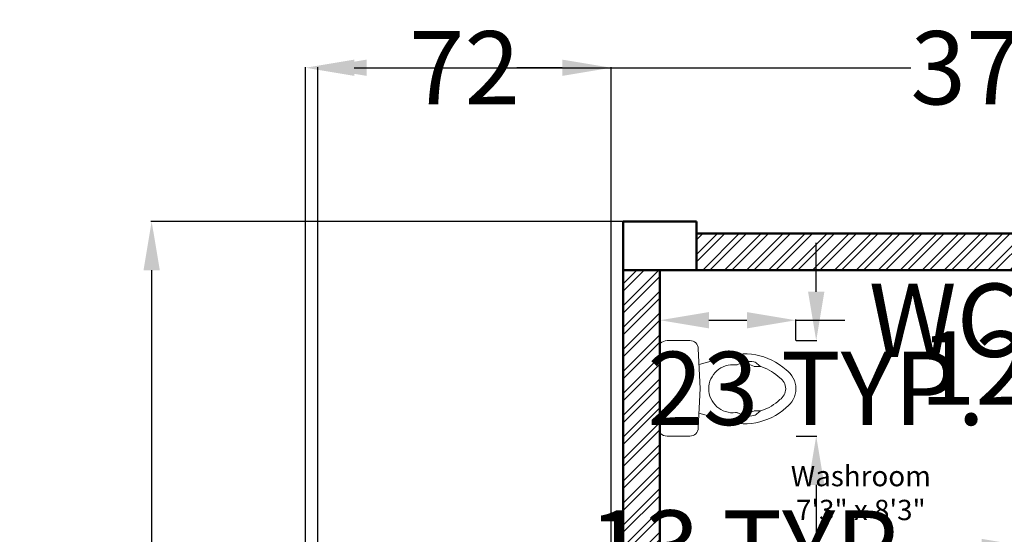
# Model space of a CAD drawing. Units: inches. Extents: x -90 to 536, y -553 to 299.
# Tile 21 of 27: x -35 to 207, y 173 to 299. Entities that reach past the tile are written whole.
import ezdxf

# ---------------------------------------------------------------- set-up
doc = ezdxf.new("R2010")
doc.units = ezdxf.units.IN
for name, color, linetype, lineweight in [('A-ANNO-DIMS', 2, 'Continuous', 18), ('A-AREA-IDEN', 7, 'Continuous', 18), ('A-COLS', 7, 'Continuous', 50), ('A-FLOR-FIXT', 8, 'Continuous', 18), ('A-WALL-PATT', 252, 'Continuous', 13), ('Outer Wall', 1, 'Continuous', 50)]:
    doc.layers.add(name, color=color, linetype=linetype, lineweight=lineweight)
doc.styles.get("Standard").update_dxf_attribs({"font": 'arial.ttf'})
doc.dimstyles.get("Standard").update_dxf_attribs({"dimtxt": 18, "dimasz": 12, "dimexe": 0.18, "dimexo": 0.0625, "dimgap": 0.09, "dimtad": 0, "dimtih": 1, "dimtoh": 1, "dimdec": 0, "dimzin": 0, "dimdsep": 46, "dimlunit": 3, "dimtxsty": 'Standard', "dimcen": 0.09, "dimadec": 0, "dimazin": 0, "dimtfac": 1, "dimtdec": 0, "dimtofl": 0, "dimtmove": 0, "dimatfit": 3, "dimfxl": 1, "dimtolj": 1, "dimtzin": 0, "dimarcsym": 0})

# ---------------------------------------------------------------- blocks, each defined once
blk = doc.blocks.new('A$C1308471B')
at = {"ltscale": 20}
for p, q in [((0, 0.4607), (0, 0.0186)), ((0.0354, 0.4793), (0.1495, 0.4793)), ((0.2013, 0.2397), (0.1923, 0.4384)), ((0.1957, 0.3639), (0.3109, 0.3953)), ((0.5021, 0.3528), (0.4724, 0.3528)), ((0.4982, 0.3575), (0.4822, 0.3709)), ((0.2013, 0.2397), (0.1923, 0.0409)), ((0.1959, 0.1193), (0.3109, 0.0879)), ((0.5021, 0.1304), (0.4724, 0.1304)), ((0.4982, 0.1257), (0.4822, 0.1123)), ((0.0354, 0), (0.1495, 0))]:
    blk.add_line(p, q, dxfattribs=at)
for centre, radius, start, end in [((0.006, 0.4607), 0.006, 136.5269, 180), ((0.0354, 0.4328), 0.0465, 90, 136.5269), ((0.1495, 0.4365), 0.0429, 2.5755, 90), ((0.4248, 0.1104), 0.3068, 47.4135, 111.7924), ((0.3654, 0.2416), 0.1206, 83.3523, 180), ((0.3823, 0.3868), 0.0255, 263.3523, 298.5742), ((0.4494, 0.2636), 0.1148, 79.3968, 118.5742), ((0.405, 0.2159), 0.153, 63.502, 90.4522), ((0.4658, 0.3513), 0.0255, 50, 79.3968), ((0.5146, 0.377), 0.0255, 230, 251.3881), ((0.5021, 0.3273), 0.0255, 70.3751, 90), ((0.4248, 0.1104), 0.2558, 46.612, 70.3751), ((0.5654, 0.2416), 0.065, 0, 57.2974), ((0.5654, 0.2416), 0.116, 0, 54.7115), ((0.3654, 0.2416), 0.1206, 180, 276.6477), ((0.5654, 0.2416), 0.065, 302.7026, 0), ((0.5654, 0.2416), 0.116, 305.2885, 0), ((0.4248, 0.3728), 0.2558, 289.6249, 313.388), ((0.4248, 0.3728), 0.3068, 248.2076, 312.5865), ((0.3823, 0.0964), 0.0255, 61.4258, 96.6477), ((0.4494, 0.2196), 0.1148, 241.4258, 280.6032), ((0.405, 0.2673), 0.153, 269.5478, 296.498), ((0.4658, 0.1319), 0.0255, 280.6032, 310), ((0.5146, 0.1062), 0.0255, 108.6119, 130), ((0.5021, 0.1559), 0.0255, 270, 289.6249), ((0.006, 0.0186), 0.006, 180, 223.4731), ((0.0354, 0.0465), 0.0465, 223.4731, 270), ((0.1495, 0.0429), 0.0429, 270, 357.4245)]:
    blk.add_arc(centre, radius, start, end, dxfattribs=at)
blk = doc.blocks.new('COL-12X18')
blk.add_lwpolyline([(0, 18), (12, 18), (12, 0), (0, 0)], close=True)
blk = doc.blocks.new('*D21')
at = {"layer": 'A-ANNO-DIMS', "color": 0, "lineweight": -2, "transparency": 16777216}
for p, q in [((122.13, 220.23), (122.13, 225.35)), ((134.13, 225.17), (143.49, 225.17)), ((155.49, 220.23), (155.49, 225.35)), ((155.49, 225.17), (167.49, 225.17))]:
    blk.add_line(p, q, dxfattribs=at)
at = {"layer": 'A-ANNO-DIMS', "color": 0, "transparency": 16777216}
for points in [[(134.13, 227.17), (134.13, 223.17), (122.13, 225.17)], [(143.49, 227.17), (143.49, 223.17), (155.49, 225.17)]]:
    blk.add_solid(points, dxfattribs=at)
at = {"layer": 'Defpoints', "color": 0, "transparency": 16777216}
for p in [(155.49, 225.17), (122.13, 220.17), (155.49, 220.17)]:
    blk.add_point(p, dxfattribs=at)
at = {"layer": 'A-ANNO-DIMS', "color": 0, "transparency": 16777216, "insert": (236.2, 225.17), "char_height": 18, "attachment_point": 5}
blk.add_mtext('\\A1;WC 33 TYP.', dxfattribs=at)
blk = doc.blocks.new('*D22')
at = {"layer": 'A-ANNO-DIMS', "color": 0, "lineweight": -2, "transparency": 16777216}
for p, q in [((160.49, 232.17), (160.49, 244.17)), ((155.55, 220.17), (160.67, 220.17)), ((155.55, 196.7), (160.67, 196.7)), ((160.49, 184.7), (160.49, 172.7))]:
    blk.add_line(p, q, dxfattribs=at)
at = {"layer": 'A-ANNO-DIMS', "color": 0, "transparency": 16777216}
for points in [[(158.49, 232.17), (162.49, 232.17), (160.49, 220.17)], [(158.49, 184.7), (162.49, 184.7), (160.49, 196.7)]]:
    blk.add_solid(points, dxfattribs=at)
at = {"layer": 'Defpoints', "color": 0, "transparency": 16777216}
for p in [(155.49, 220.17), (155.49, 196.7), (160.49, 196.7)]:
    blk.add_point(p, dxfattribs=at)
at = {"layer": 'A-ANNO-DIMS', "color": 0, "transparency": 16777216, "insert": (160.49, 208.43), "char_height": 18, "attachment_point": 5}
blk.add_mtext('\\A1;23 TYP.', dxfattribs=at)
blk = doc.blocks.new('*D24')
at = {"layer": 'A-ANNO-DIMS', "color": 0, "lineweight": -2, "transparency": 16777216}
for p, q in [((282.43, 261.45), (282.43, 273.45)), ((285.07, 249.45), (282.25, 249.45)), ((285.07, 237.45), (282.25, 237.45)), ((282.43, 225.45), (282.43, 213.45)), ((282.43, 213.45), (270.43, 213.45))]:
    blk.add_line(p, q, dxfattribs=at)
at = {"layer": 'A-ANNO-DIMS', "color": 0, "transparency": 16777216}
for points in [[(280.43, 261.45), (284.43, 261.45), (282.43, 249.45)], [(280.43, 225.45), (284.43, 225.45), (282.43, 237.45)]]:
    blk.add_solid(points, dxfattribs=at)
at = {"layer": 'Defpoints', "color": 0, "transparency": 16777216}
for p in [(285.13, 249.45), (282.43, 237.45), (285.13, 237.45)]:
    blk.add_point(p, dxfattribs=at)
at = {"layer": 'A-ANNO-DIMS', "color": 0, "transparency": 16777216, "insert": (227.38, 213.45), "char_height": 18, "attachment_point": 5}
blk.add_mtext('\\A1;12 TYP.', dxfattribs=at)
blk = doc.blocks.new('*D26')
at = {"layer": 'A-ANNO-DIMS', "color": 0, "lineweight": -2, "transparency": 16777216}
for p, q in [((201.13, 169.45), (189.13, 169.45)), ((213.13, 167), (213.13, 169.63)), ((226.43, 167), (226.43, 169.63)), ((238.43, 169.45), (250.43, 169.45))]:
    blk.add_line(p, q, dxfattribs=at)
at = {"layer": 'A-ANNO-DIMS', "color": 0, "transparency": 16777216}
for points in [[(201.13, 171.45), (201.13, 167.45), (213.13, 169.45)], [(238.43, 171.45), (238.43, 167.45), (226.43, 169.45)]]:
    blk.add_solid(points, dxfattribs=at)
at = {"layer": 'Defpoints', "color": 0, "transparency": 16777216}
for p in [(213.13, 169.45), (213.13, 166.94), (226.43, 166.94)]:
    blk.add_point(p, dxfattribs=at)
at = {"layer": 'A-ANNO-DIMS', "color": 0, "transparency": 16777216, "insert": (146.08, 169.45), "char_height": 18, "attachment_point": 5}
blk.add_mtext('\\A1;13 TYP.', dxfattribs=at)
blk = doc.blocks.new('*D32')
at = {"layer": 'A-ANNO-DIMS', "color": 0, "lineweight": -2, "transparency": 16777216}
for p, q in [((59.26, 152.75), (47.26, 152.75)), ((65.58, 142.54), (59.26, 152.75)), ((69.35, 130.76), (72.05, 132.44)), ((78.69, 115.67), (81.39, 117.34)), ((87.55, 107.05), (93.87, 96.84))]:
    blk.add_line(p, q, dxfattribs=at)
at = {"layer": 'A-ANNO-DIMS', "color": 0, "transparency": 16777216}
for points in [[(67.28, 143.6), (63.88, 141.49), (71.89, 132.34)], [(89.25, 108.1), (85.85, 105.99), (81.24, 117.25)]]:
    blk.add_solid(points, dxfattribs=at)
at = {"layer": 'Defpoints', "color": 0, "transparency": 16777216}
for p in [(69.29, 130.73), (71.89, 132.34), (78.63, 115.64)]:
    blk.add_point(p, dxfattribs=at)
at = {"layer": 'A-ANNO-DIMS', "color": 0, "transparency": 16777216, "insert": (4.21, 152.75), "char_height": 18, "attachment_point": 5}
blk.add_mtext('\\A1;18 TYP.', dxfattribs=at)
blk = doc.blocks.new('*D53')
at = {"layer": 'A-ANNO-DIMS', "color": 0, "lineweight": -2, "transparency": 16777216}
for p, q in [((35.09, 103.75), (35.09, 287.38)), ((47.09, 287.2), (183.7, 287.2)), ((395.13, 287.2), (258.52, 287.2)), ((407.13, -63.49), (407.13, 287.38))]:
    blk.add_line(p, q, dxfattribs=at)
at = {"layer": 'A-ANNO-DIMS', "color": 0, "transparency": 16777216}
for points in [[(47.09, 289.2), (47.09, 285.2), (35.09, 287.2)], [(395.13, 289.2), (395.13, 285.2), (407.13, 287.2)]]:
    blk.add_solid(points, dxfattribs=at)
at = {"layer": 'Defpoints', "color": 0, "transparency": 16777216}
for p in [(407.13, 287.2), (35.09, 103.69), (407.13, -63.55)]:
    blk.add_point(p, dxfattribs=at)
at = {"layer": 'A-ANNO-DIMS', "color": 0, "transparency": 16777216, "insert": (221.11, 287.2), "char_height": 18, "attachment_point": 5}
blk.add_mtext('\\A1;372.04', dxfattribs=at)
blk = doc.blocks.new('*D54')
at = {"layer": 'A-ANNO-DIMS', "color": 0, "lineweight": -2, "transparency": 16777216}
for p, q in [((113.07, 249.45), (-2.85, 249.45)), ((-2.67, 237.45), (-2.67, -117.77)), ((-2.67, -491.55), (-2.67, -136.34)), ((38.07, -503.55), (-2.85, -503.55))]:
    blk.add_line(p, q, dxfattribs=at)
at = {"layer": 'A-ANNO-DIMS', "color": 0, "transparency": 16777216}
for points in [[(-4.67, 237.45), (-0.67, 237.45), (-2.67, 249.45)], [(-4.67, -491.55), (-0.67, -491.55), (-2.67, -503.55)]]:
    blk.add_solid(points, dxfattribs=at)
at = {"layer": 'Defpoints', "color": 0, "transparency": 16777216}
for p in [(-2.67, 249.45), (113.13, 249.45), (38.13, -503.55)]:
    blk.add_point(p, dxfattribs=at)
at = {"layer": 'A-ANNO-DIMS', "color": 0, "transparency": 16777216, "insert": (-2.67, -127.05), "char_height": 18, "attachment_point": 5}
blk.add_mtext('\\A1;753', dxfattribs=at)
blk = doc.blocks.new('*D63')
at = {"layer": 'A-ANNO-DIMS', "color": 0, "lineweight": -2, "transparency": 16777216}
for p, q in [((38.13, 143.51), (38.13, 287.38)), ((50.13, 287.2), (61.32, 287.2)), ((98.13, 287.2), (86.95, 287.2)), ((110.13, 143.51), (110.13, 287.38))]:
    blk.add_line(p, q, dxfattribs=at)
at = {"layer": 'A-ANNO-DIMS', "color": 0, "transparency": 16777216}
for points in [[(50.13, 289.2), (50.13, 285.2), (38.13, 287.2)], [(98.13, 289.2), (98.13, 285.2), (110.13, 287.2)]]:
    blk.add_solid(points, dxfattribs=at)
at = {"layer": 'Defpoints', "color": 0, "transparency": 16777216}
for p in [(110.13, 287.2), (38.13, 143.45), (110.13, 143.45)]:
    blk.add_point(p, dxfattribs=at)
at = {"layer": 'A-ANNO-DIMS', "color": 0, "transparency": 16777216, "insert": (74.13, 287.2), "char_height": 18, "attachment_point": 5}
blk.add_mtext('\\A1;72', dxfattribs=at)

msp = doc.modelspace()

# ---------------------------------------------------------------- hatches: boundary and pattern name
at = {"layer": 'A-WALL-PATT'}
h = msp.add_hatch(dxfattribs=at)
h.set_pattern_fill('ANSI32', color=256, scale=0.4)
h.set_pattern_definition([(45, (-88.8105, -603.6155), (-2.694077, 2.694077), []), (45, (-87.0145, -603.6155), (-2.694077, 2.694077), [])])
h.paths.add_polyline_path([(285.1317, 246.4462), (131.1317, 246.4462), (131.1317, 237.4462), (285.1317, 237.4462)])
h.paths.add_polyline_path([(122.1317, 237.4462), (113.1317, 237.4462), (113.1317, 152.4462), (122.1317, 152.4462), (122.1317, 166.4704)])
h.paths.add_polyline_path([(303.1317, 237.4462), (294.1317, 237.4462), (294.1317, 152.4462), (303.1317, 152.4462)])
h.paths.add_polyline_path([(47.1317, 91.9277), (38.1317, 91.9277), (38.1317, -6.5538), (77.1317, -6.5538), (77.1317, 2.4462), (70.5655, 2.4462), (47.1317, 2.4462)])
h.paths.add_polyline_path([(83.052, -61.5538), (47.1317, -61.5538), (47.1317, -24.5538), (38.1317, -24.5538), (38.1317, -70.5538), (74.052, -70.5538), (74.052, -223.5538), (38.1317, -223.5538), (38.1317, -503.5538), (92.1317, -503.5538), (92.1317, -437.5538), (191.1317, -437.5538), (191.1317, -428.5538), (83.1317, -428.5538), (83.1317, -494.5538), (47.1317, -494.5538), (47.1317, -232.5538), (83.052, -232.5538), (83.052, -70.5538)])
h.paths.add_polyline_path([(407.1317, -63.5538), (381.1317, -63.5538), (381.1317, 91.9277), (372.1317, 91.9277), (372.1317, 32.8805), (372.1317, -63.5538), (306.5745, -63.5538), (237.1317, -63.5538), (237.1317, -38.5538), (233.1317, -38.5538), (233.1317, -71.5538), (398.1317, -71.5538), (398.1317, -152.5538), (233.1317, -152.5538), (233.1317, -161.5538), (398.1317, -161.5538), (398.1317, -368.5538), (233.1317, -368.5538), (233.1317, -377.5538), (407.1317, -377.5538), (407.1317, -161.5538)])
h.paths.add_polyline_path([(261.1317, -422.5538), (252.1317, -422.5538), (252.1317, -428.5538), (233.1317, -428.5538), (233.1317, -437.5538), (261.1317, -437.5538)])
h.paths.add_polyline_path([(191.1317, -368.5538), (180.1317, -368.5538), (180.1317, -335.5538), (131.5919, -335.5538), (131.5919, -344.5538), (171.1317, -344.5538), (171.1317, -392.5538), (180.1317, -392.5538), (180.1317, -377.5538), (191.1317, -377.5538)], flags=17)
h.paths.add_polyline_path([(180.1317, -223.5538), (152.1317, -223.5538), (152.1317, -227.5538), (176.1317, -227.5538), (176.1317, -335.5538), (180.1317, -335.5538)], flags=17)
h.paths.add_polyline_path([(131.5919, -335.5538), (83.1317, -335.5538), (83.1317, -339.5538), (83.1317, -392.5538), (87.1317, -392.5538), (87.1317, -339.5538), (131.5919, -339.5538)], flags=17)
h.paths.add_polyline_path([(197.1317, 2.4462), (77.1317, 2.4462), (77.1317, -1.5538), (113.1317, -1.5538), (113.1317, -71.5538), (181.1317, -71.5538), (181.1317, -67.5538), (117.1317, -67.5538), (117.1317, -1.5538), (177.1317, -1.5538), (177.1317, -37.5538), (181.1317, -37.5538), (181.1317, -1.5538), (197.1317, -1.5538)])
h.paths.add_polyline_path([(173.1317, 138.4462), (122.1317, 138.4462), (122.1317, 134.4462), (173.1317, 134.4462)])
h.paths.add_polyline_path([(213.1317, 237.4462), (209.1317, 237.4462), (209.1317, 134.4462), (233.1317, 134.4462), (233.1317, 68.8889), (233.1317, -2.5538), (237.1317, -2.5538), (237.1317, 134.4462), (258.1317, 134.4462), (258.1317, 138.4462), (213.1317, 138.4462)])

# ---------------------------------------------------------------- linework, layer by layer
at = {"layer": 'Outer Wall'}
for p, q in [((113.1317, 152.4462), (113.1317, 246.4462)), ((131.1317, 246.4462), (285.1317, 246.4462)), ((122.1317, 138.4462), (122.1317, 237.4462)), ((122.1317, 237.4462), (294.1317, 237.4462))]:
    msp.add_line(p, q, dxfattribs=at)

# ---------------------------------------------------------------- block references
at = {"layer": 'A-COLS', "rotation": 269.9999999999999}
msp.add_blockref('COL-12X18', (113.1317, 249.4462), dxfattribs=at)
at = {"layer": 'A-FLOR-FIXT', "xscale": -48.95497407897215, "yscale": 48.95497407897215, "zscale": 48.95497407897215, "rotation": 180}
msp.add_blockref('A$C1308471B', (122.1317, 220.1654), dxfattribs=at)

# ---------------------------------------------------------------- texts
at = {"layer": 'A-AREA-IDEN', "insert": (189.0592, 189.3861), "char_height": 5, "attachment_point": 3}
msp.add_mtext_dynamic_manual_height_columns('\\pxqc;{\\fTimes New Roman|b0|i0|c0|p18;Washroom\\P7\'3" x 8\'3"}', width=35.23368, gutter_width=12.5, heights=[0], dxfattribs=at)

# ---------------------------------------------------------------- dimensions: what is measured, and where the dimension line sits
at = {"layer": 'A-ANNO-DIMS'}
for base, p1, p2, override, picture, middle in [((407.1317, 287.2012), (35.0873, 103.6916), (407.1317, -63.5538), {"dimdec": 2, "dimlfac": 1, "dimrnd": 0, "dimzin": 0, "dimdsep": 46, "dimlunit": 2}, '*D53', (221.1095, 287.2012)), ((110.1317, 287.2012), (38.1317, 143.4462), (110.1317, 143.4462), {"dimdec": 0, "dimlfac": 1, "dimrnd": 0, "dimzin": 0, "dimdsep": 46, "dimlunit": 2}, '*D63', (74.1317, 287.2012))]:
    dim = msp.add_linear_dim(base=base, p1=p1, p2=p2, dimstyle='Standard', override=override, dxfattribs=at)
    dim.commit()
    dim.dimension.update_dxf_attribs({"geometry": picture, "text_midpoint": middle})
for base, p1, p2, angle, picture, middle in [((282.4317, 237.4462), (285.1317, 249.4462), (285.1317, 237.4462), 270, '*D24', (227.3799, 213.4462)), ((160.492, 196.6989), (155.4885, 220.1654), (155.4885, 196.6989), 270, '*D22', (160.492, 208.4321)), ((213.1317, 169.4531), (226.4312, 166.9352), (213.1317, 166.9352), 180, '*D26', (146.0799, 169.4531)), ((71.8939, 132.3414), (78.6344, 115.6404), (69.2932, 130.7316), 121.756702, '*D32', (4.2106, 152.7484))]:
    dim = msp.add_linear_dim(base=base, p1=p1, p2=p2, angle=angle, text='<> TYP.', dimstyle='Standard', override={"dimdec": 0, "dimlfac": 1, "dimrnd": 0, "dimzin": 0, "dimdsep": 46, "dimlunit": 2}, dxfattribs=at)
    dim.commit()
    dim.dimension.update_dxf_attribs({"geometry": picture, "text_midpoint": middle})
dim = msp.add_linear_dim(base=(155.4885, 225.1689), p1=(122.1317, 220.1654), p2=(155.4885, 220.1654), text='WC <> TYP.', dimstyle='Standard', override={"dimdec": 0, "dimlfac": 1, "dimrnd": 0, "dimzin": 0, "dimdsep": 46, "dimlunit": 2}, dxfattribs=at)
dim.commit()
dim.dimension.update_dxf_attribs({"geometry": '*D21', "text_midpoint": (236.1958, 225.1689)})
dim = msp.add_linear_dim(base=(-2.6677, 249.4462), p1=(38.1317, -503.5538), p2=(113.1317, 249.4462), angle=90, dimstyle='Standard', override={"dimdec": 0, "dimlfac": 1, "dimrnd": 0, "dimzin": 0, "dimdsep": 46, "dimlunit": 2}, dxfattribs=at)
dim.commit()
dim.dimension.update_dxf_attribs({"geometry": '*D54', "text_midpoint": (-2.6677, -127.0538)})

doc.saveas('drawing.dxf')
